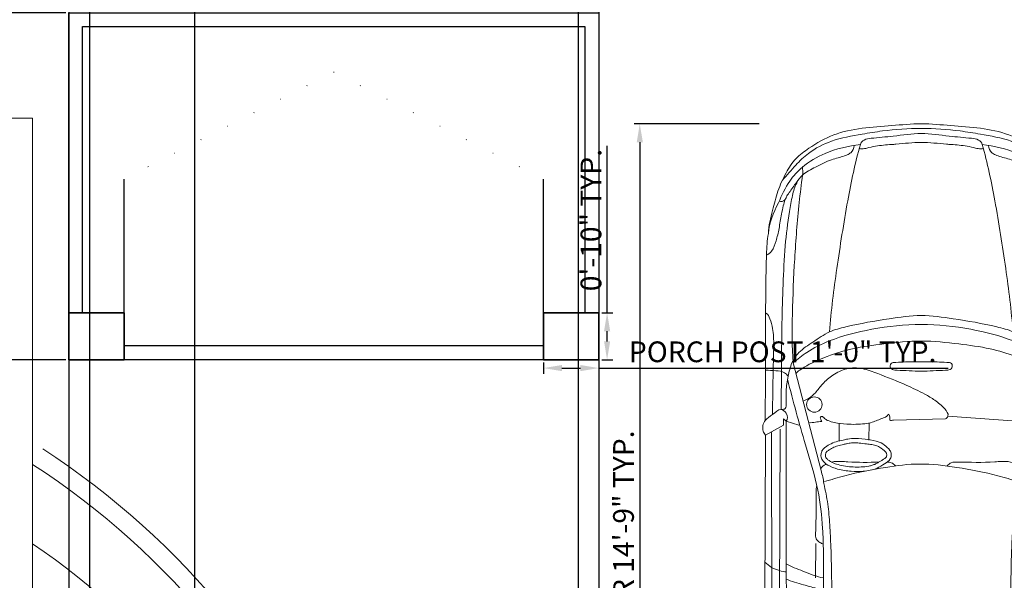
# Model space of a CAD drawing. Units: inches. Extents: x 1239 to 2276906, y 2273 to 321338.
# Tile 9 of 23: x 1541 to 1754, y 2507 to 2629. Entities that reach past the tile are written whole.
import ezdxf

# ---------------------------------------------------------------- set-up
doc = ezdxf.new("R2010")
doc.units = ezdxf.units.IN
doc.linetypes.add('DOT', pattern=[6.35, 0, -6.35])
for name, color, linetype, lineweight in [('A-ANNO-DIMS', 2, 'Continuous', 18), ('A-COLS', 7, 'Continuous', 35), ('A-FLOR-PORCH', 7, 'Continuous', 25), ('A-FLOR-PORCH-OVHD', 8, 'DOT', 18), ('C-PRKG', 8, 'Continuous', 13), ('L-PLNT', 94, 'Continuous', 13)]:
    doc.layers.add(name, color=color, linetype=linetype, lineweight=lineweight)
doc.styles.get("Standard").update_dxf_attribs({"font": 'arial.ttf'})
doc.dimstyles.new('ISO-25', dxfattribs={"dimtxt": 4.5, "dimasz": 4, "dimexe": 1.25, "dimexo": 0.625, "dimtad": 1, "dimdec": 1, "dimlunit": 3, "dimtxsty": 'Standard', "dimcen": 2.5, "dimadec": 0, "dimazin": 0, "dimtfac": 1, "dimtdec": 1, "dimtmove": 0, "dimatfit": 3, "dimfxl": 1, "dimarcsym": 0})

# ---------------------------------------------------------------- blocks, each defined once
blk = doc.blocks.new('A$C242571DA')
for p, q in [((1714.3, 1732.5), (3817.1, 1739.9)), ((1659.9, 1632), (1714.3, 1732.5)), ((1699.9, 1699.4), (2984.7, 1695.8)), ((1638.3, 1618.5), (1625.1, 1632)), ((1625.1, 1632), (1659.9, 1632)), ((1681.8, 1651.6), (2695.2, 1655.3)), ((1317.4, 1579.7), (1909.8, 1424.9)), ((1638.3, 1618.5), (2503.3, 1618.5)), ((1659.9, 1548.1), (1638.3, 1618.5)), ((2503.3, 1618.5), (2861.6, 1607.5)), ((3007.2, 1526.5), (2808.1, 1525.2)), ((1644, 1489.1), (1610.4, 1020.2)), ((2311.9, 1454.3), (2500.6, 1456.9)), ((3474.6, 1401.1), (3474.6, 843)), ((4315.2, 1398), (4377.3, 1370.5)), ((1626.1, 1006.5), (1632.8, 719.7)), ((3474.6, 345.6), (3474.6, 903.8)), ((1740.2, 584.9), (1649.3, 586.9)), ((1746.1, 420.6), (1649.3, 420.6)), ((4315.2, 348.7), (4377.3, 376.3)), ((1317.4, 167), (1909.8, 321.9)), ((2311.9, 292.5), (2500.6, 289.8)), ((3007.2, 220.3), (2808.1, 221.6)), ((1659.9, 198.7), (1638.3, 128.2)), ((1638.3, 128.2), (1625.1, 114.7)), ((1625.1, 114.7), (1659.9, 114.7)), ((1638.3, 128.2), (2503.3, 128.2)), ((1659.9, 114.7), (1714.3, 14.2)), ((2503.3, 128.2), (2861.6, 139.2)), ((1681.8, 95.1), (2695.2, 91.4)), ((1699.9, 47.3), (2984.7, 51)), ((1714.3, 14.2), (3817.1, 6.9))]:
    blk.add_line(p, q)
for centre in [(1546.4, 1462.5), (1546.4, 284.2)]:
    blk.add_ellipse(centre, major_axis=(0, 42.9), ratio=0.983266, start_param=4.712389, end_param=10.995574)
for points, knots in [([(1714.3, 1732.5), (1707.7, 1737.6), (1683.3, 1753), (1628.7, 1741.2), (1605.6, 1691.5), (1561.7, 1652.4), (1594.1, 1610.3), (1627.9, 1608.3), (1638.3, 1618.5)], [0, 0, 0, 0, 0.024864, 0.0846267, 0.1362471, 0.1900683, 0.2245199, 0.2681841, 0.2681841, 0.2681841, 0.2681841]), ([(3356.5, 1739.4), (3354.9, 1719.2), (3360.8, 1678.2), (3324, 1631.5), (3255.4, 1544.3), (3187.1, 1476.2), (3125.2, 1432.2)], [0, 0, 0, 0, 0.0597371, 0.1139981, 0.1672498, 0.3938869, 0.3938869, 0.3938869, 0.3938869]), ([(3745.3, 1736.8), (3748.5, 1730.1), (3764.2, 1717.1), (3811.5, 1698.6), (3894.7, 1686.7), (4002.9, 1663.2), (4107.9, 1648.7), (4195.8, 1638.3), (4258.6, 1603.2), (4302.1, 1549.7), (4339.9, 1483.8), (4365.2, 1407.6), (4389.6, 1324.4), (4397.9, 1266.9), (4401.8, 1235.2)], [0, 0, 0, 0, 0.0219205, 0.0572122, 0.1522539, 0.2718866, 0.3894011, 0.4710097, 0.5346344, 0.5986698, 0.6733118, 0.758696, 0.8351341, 0.9293726, 0.9293726, 0.9293726, 0.9293726]), ([(3817.1, 1739.9), (3833.2, 1729.7), (3882.9, 1718.2), (3973.3, 1695.2), (4085.1, 1680.5), (4193.8, 1662.8), (4280.6, 1644.3), (4343.9, 1598.1), (4390, 1540.3), (4427.4, 1448.7), (4457.8, 1336.6), (4475.7, 1233.4), (4478.4, 1175.1), (4479.3, 1161.6)], [0, 0, 0, 0, 0.056668, 0.14946, 0.28161, 0.392935, 0.481686, 0.542967, 0.622845, 0.69797, 0.833643, 0.965665, 1.00577, 1.00577, 1.00577, 1.00577]), ([(0, 873.4), (0, 927.8), (15.6, 1088.6), (25.5, 1309.8), (120.7, 1476.4), (189.2, 1569), (273.5, 1623.1), (369.9, 1666.3), (483, 1694.7), (561.3, 1714.9), (604.6, 1715.7)], [0, 0, 0, 0, 0.16039, 0.479033, 0.632967, 0.722015, 0.817474, 0.927562, 1.03733, 1.167094, 1.167094, 1.167094, 1.167094]), ([(604.6, 1715.7), (545.5, 1714.5), (448.5, 1664.6), (320.8, 1610.6), (225.4, 1521.2), (147.3, 1390.5), (121.7, 1275.2), (113.6, 1208.7)], [0, 0, 0, 0, 0.1772572, 0.3124951, 0.4151678, 0.5597243, 0.7575412, 0.7575412, 0.7575412, 0.7575412]), ([(722.7, 1726.6), (720.8, 1714.9), (694.5, 1689.9), (643, 1671.8), (573.6, 1655.4), (508.5, 1647), (455.2, 1634.7), (428.7, 1627.3), (416.9, 1624.1)], [0, 0, 0, 0, 0.034703, 0.0959761, 0.1659336, 0.2471559, 0.2929944, 0.3295918, 0.3295918, 0.3295918, 0.3295918]), ([(604.6, 1715.7), (642.1, 1723.4), (788.5, 1729.2), (1039.3, 1732.2), (1344.5, 1729.9), (1542, 1733.1), (1633.8, 1733.7)], [0, 0, 0, 0, 0.114897, 0.437061, 0.754269, 1.029686, 1.029686, 1.029686, 1.029686]), ([(1043.6, 1729.2), (1048.6, 1717.9), (1080.9, 1704.2), (1138.6, 1687.6), (1237.7, 1685.6), (1394.7, 1691.3), (1521.7, 1692.4), (1601.5, 1692.7)], [0, 0, 0, 0, 0.0364992, 0.0923739, 0.1867837, 0.3273982, 0.5667068, 0.5667068, 0.5667068, 0.5667068]), ([(1356.8, 1732.2), (1357.1, 1712.8), (1360, 1678.8), (1363.9, 1630.5), (1383.3, 1613.5), (1391, 1607.2)], [0, 0, 0, 0, 1.462159, 2.651105, 3.386321, 3.386321, 3.386321, 3.386321]), ([(2414.7, 1735), (2424.9, 1723.3), (2447.2, 1698.8), (2461.2, 1657.6), (2468.1, 1629), (2468, 1616.1)], [1.808086, 1.808086, 1.808086, 1.808086, 2.918874, 4.131288, 5.10151, 5.10151, 5.10151, 5.10151]), ([(2984.7, 1695.8), (3051, 1695.6), (3172.1, 1691.3), (3367.4, 1677.6), (3575.2, 1664.3), (3788.2, 1643.6), (3968, 1628.1), (4103.8, 1616.8), (4203.6, 1578.1), (4271.8, 1519.5), (4300.6, 1452.1), (4341.7, 1305.3), (4361.8, 1111.2), (4367.5, 936.8), (4367.5, 873.4)], [0, 0, 0, 0, 0.198873, 0.363323, 0.587433, 0.823543, 1.004622, 1.129816, 1.230113, 1.320655, 1.388577, 1.443334, 1.771447, 1.958652, 1.958652, 1.958652, 1.958652]), ([(310.7, 1637.3), (282.5, 1613.7), (230.1, 1569.9), (148.7, 1486.2), (84.8, 1361.3), (60, 1219), (32.6, 1054.3), (25.1, 944.9), (25.1, 873.4)], [0, 0, 0, 0, 0.1095129, 0.2035347, 0.3452507, 0.5161382, 0.6275464, 0.8383798, 0.8383798, 0.8383798, 0.8383798]), ([(426.8, 1656.7), (428.5, 1646.6), (426.9, 1625), (399.8, 1616.6), (368.1, 1593.9), (328, 1564.6), (271.6, 1523.9), (237, 1451.9), (196.2, 1376.7), (183.8, 1314.9), (170, 1279.6), (157.2, 1254.2), (133.3, 1244.4), (118.6, 1242.9)], [0, 0, 0, 0, 0.0304541, 0.0502818, 0.0786089, 0.1479133, 0.1986294, 0.2831705, 0.3780326, 0.4523267, 0.4667809, 0.4902599, 0.5347198, 0.5347198, 0.5347198, 0.5347198]), ([(323.7, 1557.5), (344.8, 1571.9), (400.4, 1585.1), (516, 1606.8), (680.3, 1625.8), (885.4, 1635.7), (1116.8, 1642.2), (1346.1, 1644.2), (1504.7, 1644.7), (1574, 1645.7)], [0, 0, 0, 0, 0.076148, 0.165903, 0.355672, 0.569871, 0.782325, 1.050047, 1.257936, 1.257936, 1.257936, 1.257936]), ([(1574, 1645.7), (1572.9, 1638), (1574.1, 1622), (1559.9, 1618.7), (1555.2, 1617.8)], [0, 0, 0, 0, 0.02274132, 0.03717479, 0.03717479, 0.03717479, 0.03717479]), ([(2695.2, 1655.3), (2829.9, 1655.3), (3041.2, 1651.4), (3351.3, 1630.7), (3527.5, 1623.2), (3626.6, 1612)], [0, 0, 0, 0, 0.4042759, 0.6333827, 0.9326252, 0.9326252, 0.9326252, 0.9326252]), ([(1317.4, 1579.7), (1227.8, 1586.1), (1036, 1584.8), (741.2, 1572.5), (486.1, 1553.3), (333.3, 1534.3), (283.3, 1528.5)], [0, 0, 0, 0, 0.269375, 0.574535, 0.885339, 1.036319, 1.036319, 1.036319, 1.036319]), ([(1555.2, 1617.8), (1527.7, 1617.8), (1472.5, 1620.4), (1392.7, 1608.8), (1318.5, 1591), (1249.4, 1545.5), (1201.4, 1466.7), (1142.8, 1385.7), (1104.8, 1240.4), (1076, 1072.3), (1056.4, 932.4), (1056.4, 873.4)], [0, 0, 0, 0, 0.082256, 0.165174, 0.241383, 0.30939, 0.405348, 0.511507, 0.603349, 0.843635, 1.017671, 1.017671, 1.017671, 1.017671]), ([(1317.4, 1579.7), (1296.6, 1555.5), (1247.9, 1494.4), (1177.6, 1350.5), (1124.2, 1137.4), (1105.5, 964.9), (1105.5, 873.4)], [0, 0, 0, 0, 0.0947759, 0.2311242, 0.4700259, 0.7400315, 0.7400315, 0.7400315, 0.7400315]), ([(3535.9, 1563.1), (3520.1, 1550.9), (3484.4, 1526.1), (3408.2, 1510.9), (3323.4, 1473.1), (3207.9, 1445), (3072.6, 1422.2), (2866.9, 1404.6), (2626.4, 1412.9), (2396.7, 1410.8), (2200.9, 1416.9), (2001.3, 1438.2), (1732.1, 1525.9), (1527.9, 1578.9), (1407.5, 1610.7)], [0, 0, 0, 0, 0.05975, 0.126928, 0.230034, 0.336675, 0.482225, 0.641324, 0.954906, 1.203173, 1.330375, 1.542773, 1.802261, 2.175545, 2.175545, 2.175545, 2.175545]), ([(2424, 1618.7), (2441.5, 1589.9), (2464.2, 1518.9), (2495.4, 1450.9), (2501.6, 1411.3)], [0, 0, 0, 0, 0.1000351, 0.2184418, 0.2184418, 0.2184418, 0.2184418]), ([(2507.7, 1618.4), (2521, 1587.7), (2536.6, 1527.1), (2559.6, 1458.5), (2563.3, 1420.6), (2563.8, 1411.4)], [0, 0, 0, 0, 2.528586, 4.711885, 5.408215, 5.408215, 5.408215, 5.408215]), ([(2861.6, 1607.5), (2921.1, 1607.3), (3047.2, 1600.8), (3191.4, 1602), (3356.6, 1584.1), (3498.3, 1570.6), (3623.2, 1549.4), (3664.1, 1533.3)], [0, 0, 0, 0, 0.1783018, 0.3787173, 0.431954, 0.6762374, 0.8077184, 0.8077184, 0.8077184, 0.8077184]), ([(3248.1, 1545.2), (3226.9, 1550.4), (3176.1, 1562.1), (3113.7, 1592.9), (3052.6, 1605.3), (3010.4, 1578.8), (3010.3, 1545.3), (3010.3, 1515.9), (3033.7, 1500.1), (3052.6, 1465.2), (3078.9, 1443.5), (3084, 1424.4)], [0, 0, 0, 0, 0.0655106, 0.1550445, 0.2094604, 0.2438604, 0.287164, 0.3001388, 0.3275984, 0.3616951, 0.4200969, 0.4200969, 0.4200969, 0.4200969]), ([(3319, 1587.1), (3303.3, 1568.1), (3256.9, 1516.7), (3206.7, 1467.3), (3171.4, 1439.5)], [0, 0, 0, 0, 1.868162, 5.271297, 5.271297, 5.271297, 5.271297]), ([(3626.6, 1612), (3702.5, 1609.1), (3826.2, 1596.8), (3991.4, 1583.2), (4111.7, 1562.4), (4212.2, 1522.7), (4290.4, 1488), (4300.7, 1447.5)], [0, 0, 0, 0, 0.2277977, 0.3719478, 0.4996814, 0.5863441, 0.709615, 0.709615, 0.709615, 0.709615]), ([(1372.8, 1563.1), (1357.2, 1545), (1321.6, 1490.1), (1277, 1385.7), (1232.8, 1244.2), (1211.1, 1069.4), (1196.8, 942.4), (1196.8, 873.4)], [0, 0, 0, 0, 0.0708922, 0.1925846, 0.3348457, 0.5072814, 0.7109928, 0.7109928, 0.7109928, 0.7109928]), ([(2808.1, 1525.2), (2791.9, 1525.1), (2751.9, 1519.7), (2710.6, 1472.6), (2690, 1431.1), (2690.5, 1409.6)], [0, 0, 0, 0, 0.0486628, 0.1144515, 0.1777721, 0.1777721, 0.1777721, 0.1777721]), ([(3275.5, 1532.8), (3287.5, 1528.3), (3299.8, 1504.9), (3308.4, 1482.5), (3311.7, 1472.6)], [0, 0, 0, 0, 0.983949, 1.771691, 1.771691, 1.771691, 1.771691]), ([(3372.2, 1495.3), (3354.4, 1496.8), (3316, 1494.7), (3291.6, 1525.8), (3275.5, 1532.8)], [0, 0, 0, 0, 0.0535488, 0.1060573, 0.1060573, 0.1060573, 0.1060573]), ([(3664.1, 1533.3), (3687, 1526), (3734.8, 1502.3), (3816.7, 1444.8), (3884.1, 1342.9), (3925.1, 1239.9), (3937.3, 1177), (3940.4, 1157.6)], [0, 0, 0, 0, 0.0720749, 0.1581284, 0.2958089, 0.4262456, 0.4842292, 0.4842292, 0.4842292, 0.4842292]), ([(1898.5, 1426.2), (1889, 1420.6), (1871, 1397.2), (1856.4, 1345.2), (1867.7, 1233.5), (1864.3, 1132.3), (1863, 1038.5), (1876.9, 1022.3), (1884.5, 1015.7)], [0, 0, 0, 0, 0.842998, 2.122875, 3.997599, 9.174838, 10.012722, 10.751336, 10.751336, 10.751336, 10.751336]), ([(1909.8, 1424.9), (1933.5, 1418.7), (1995.6, 1407.6), (2094.4, 1385.8), (2211.8, 1377.1), (2419, 1366.9), (2704.7, 1366.5), (3032.7, 1354.2), (3316.2, 1371), (3558.7, 1415.9), (3789.1, 1461.7), (4028.9, 1452.9), (4196.2, 1455.2), (4292.7, 1447.9), (4300.7, 1447.5)], [0, 0, 0, 0, 0.073325, 0.188896, 0.303039, 0.425821, 0.811242, 1.159737, 1.41058, 1.660623, 1.899627, 2.11145, 2.377727, 2.401703, 2.401703, 2.401703, 2.401703]), ([(1997.2, 1450.5), (2039.7, 1454.5), (2126.7, 1451.9), (2219.8, 1454.5), (2287.1, 1456.9), (2305.7, 1434.4), (2313.2, 1419.9), (2315.8, 1413.5)], [0, 0, 0, 0, 3.267856, 6.568708, 7.399663, 8.099385, 8.621705, 8.621705, 8.621705, 8.621705]), ([(113.6, 1208.7), (215.2, 1238.6), (443.2, 1284.9), (788, 1338.7), (1029.5, 1370.7), (1146.4, 1378.6)], [0, 0, 0, 0, 0.317374, 0.69576, 1.04714, 1.04714, 1.04714, 1.04714]), ([(1969.6, 1407.3), (1960.5, 1369.8), (1927, 1259.1), (1890.9, 1078.4), (1874.3, 933), (1874.3, 864.4)], [0, 0, 0, 0, 0.1139079, 0.3411539, 0.543502, 0.543502, 0.543502, 0.543502]), ([(3231.5, 1368.3), (3240.8, 1356.2), (3253.1, 1315.7), (3271.9, 1240.7), (3297.9, 1127.9), (3310.5, 974.6), (3311.2, 858.3), (3311.6, 794.4)], [0, 0, 0, 0, 0.0451009, 0.1211996, 0.2308505, 0.385263, 0.5739042, 0.5739042, 0.5739042, 0.5739042]), ([(3294.8, 1174.5), (3294.8, 1207.4), (3299.6, 1249.5), (3298.3, 1303.9), (3326.3, 1329), (3363.9, 1320.7), (3399.3, 1329.3), (3422.1, 1315.7), (3430.7, 1297.9), (3438.7, 1234.2), (3439.6, 1174.4), (3434.7, 1112.2), (3418.9, 1102), (3395.9, 1098.6), (3362.6, 1100.9), (3331.1, 1096.6), (3298.8, 1107.6), (3297.3, 1140.3), (3294.8, 1160.9), (3294.8, 1174.5)], [0, 0, 0, 0, 0.0969044, 0.1295913, 0.1506192, 0.1985921, 0.2360698, 0.2557908, 0.2719711, 0.2929882, 0.44406, 0.4519132, 0.4720918, 0.4918599, 0.5228758, 0.5707096, 0.5892096, 0.6145759, 0.654681, 0.654681, 0.654681, 0.654681]), ([(113.6, 1208.7), (103.3, 1207), (83.6, 1187.6), (76.5, 1122.2), (68.2, 1017.3), (53.4, 925), (53.4, 873.4)], [0, 0, 0, 0, 0.0314754, 0.0702057, 0.1915753, 0.3439346, 0.3439346, 0.3439346, 0.3439346]), ([(135.5, 1213.1), (139.1, 1211.8), (138.4, 1193.3), (132.6, 1168.3), (118.8, 1111.9), (115.6, 1058.9), (109, 974.6), (102.4, 920.1), (102.4, 873.4)], [0, 0, 0, 0, 0.0114788, 0.0403472, 0.0875838, 0.1755608, 0.1991501, 0.3369659, 0.3369659, 0.3369659, 0.3369659]), ([(4401.8, 1235.2), (4411.9, 1185.3), (4421.6, 1065.8), (4424.1, 946.5), (4424.1, 878)], [0, 0, 0, 0, 0.1502861, 0.3522699, 0.3522699, 0.3522699, 0.3522699]), ([(3940.4, 1157.6), (3949.9, 1111), (3964.3, 1016.4), (3960.5, 921), (3959.8, 873.4)], [0, 0, 0, 0, 0.140379, 0.2808468, 0.2808468, 0.2808468, 0.2808468]), ([(3339.2, 1099), (3339.1, 1094.8), (3336.4, 1010.6), (3333.2, 926.3), (3330, 846.2)], [11.235438, 11.235438, 11.235438, 11.235438, 11.552536, 17.586883, 17.586883, 17.586883, 17.586883]), ([(1311.3, 873.4), (1311.2, 902.4), (1309.2, 950.9), (1315, 1002.2), (1314.2, 1039.4), (1332.1, 1044.9), (1345.7, 1044.2), (1356.8, 1028.5), (1359.2, 970.2), (1361.5, 917.6), (1362.9, 873.4)], [0, 0, 0, 0, 0.0857277, 0.1381048, 0.1641986, 0.1769751, 0.1890325, 0.2028129, 0.2286049, 0.3592554, 0.3592554, 0.3592554, 0.3592554]), ([(1626.1, 1006.5), (1623.5, 1013), (1603.1, 1029.4), (1559.1, 995), (1523, 951.9), (1480.3, 878.3), (1430.5, 774.3), (1385.5, 658.5), (1343.7, 551.3), (1343, 461.7), (1380.3, 386.9), (1428.2, 329.9), (1480.1, 294.6), (1509.8, 257.4), (1524.8, 232.6), (1528, 222.1)], [0, 0, 0, 0, 0.527288, 1.647451, 3.487558, 5.099073, 7.968657, 12.238313, 14.475187, 16.613757, 18.744202, 20.639343, 22.223389, 23.452731, 24.286529, 24.286529, 24.286529, 24.286529]), ([(3231.5, 378.5), (3240.8, 390.5), (3253.1, 431), (3271.9, 506.1), (3297.9, 618.9), (3310.5, 772.1), (3311.2, 888.4), (3311.6, 952.4)], [0, 0, 0, 0, 0.0451009, 0.1211996, 0.2308505, 0.385263, 0.5739042, 0.5739042, 0.5739042, 0.5739042]), ([(0, 873.4), (0, 819), (15.6, 658.1), (25.5, 437), (120.7, 270.3), (189.2, 177.8), (273.5, 123.7), (369.9, 80.4), (483, 52), (561.3, 31.9), (604.6, 31)], [0, 0, 0, 0, 0.16039, 0.479033, 0.632967, 0.722015, 0.817474, 0.927562, 1.03733, 1.167094, 1.167094, 1.167094, 1.167094]), ([(310.7, 109.5), (282.5, 133.1), (230.1, 176.9), (148.7, 260.5), (84.8, 385.5), (60, 527.8), (32.6, 692.4), (25.1, 801.9), (25.1, 873.4)], [0, 0, 0, 0, 0.1095129, 0.2035347, 0.3452507, 0.5161382, 0.6275464, 0.8383798, 0.8383798, 0.8383798, 0.8383798]), ([(113.6, 538.1), (103.3, 539.8), (83.6, 559.2), (76.5, 624.5), (68.2, 729.4), (53.4, 821.7), (53.4, 873.4)], [0, 0, 0, 0, 0.0314754, 0.0702057, 0.1915753, 0.3439346, 0.3439346, 0.3439346, 0.3439346]), ([(135.5, 533.6), (139.1, 534.9), (138.4, 553.4), (132.6, 578.4), (118.8, 634.9), (115.6, 687.8), (109, 772.2), (102.4, 826.7), (102.4, 873.4)], [0, 0, 0, 0, 0.0114788, 0.0403472, 0.0875838, 0.1755608, 0.1991501, 0.3369659, 0.3369659, 0.3369659, 0.3369659]), ([(1555.2, 129), (1527.7, 129), (1472.5, 126.3), (1392.7, 138), (1318.5, 155.7), (1249.4, 201.3), (1201.4, 280.1), (1142.8, 361.1), (1104.8, 506.4), (1076, 674.5), (1056.4, 814.4), (1056.4, 873.4)], [0, 0, 0, 0, 0.082256, 0.165174, 0.241383, 0.30939, 0.405348, 0.511507, 0.603349, 0.843635, 1.017671, 1.017671, 1.017671, 1.017671]), ([(1317.4, 167), (1296.6, 191.2), (1247.9, 252.4), (1177.6, 396.3), (1124.2, 609.4), (1105.5, 781.8), (1105.5, 873.4)], [0, 0, 0, 0, 0.0947759, 0.2311242, 0.4700259, 0.7400315, 0.7400315, 0.7400315, 0.7400315]), ([(1372.8, 183.6), (1357.2, 201.8), (1321.6, 256.7), (1277, 361), (1232.8, 502.6), (1211.1, 677.3), (1196.8, 804.3), (1196.8, 873.4)], [0, 0, 0, 0, 0.0708922, 0.1925846, 0.3348457, 0.5072814, 0.7109928, 0.7109928, 0.7109928, 0.7109928]), ([(1311.3, 873.4), (1311.2, 844.3), (1309.2, 795.8), (1315, 744.6), (1314.2, 707.4), (1332.1, 701.9), (1345.7, 702.6), (1356.8, 718.2), (1359.2, 776.6), (1361.5, 829.1), (1362.9, 873.4)], [0, 0, 0, 0, 0.0857277, 0.1381048, 0.1641986, 0.1769751, 0.1890325, 0.2028129, 0.2286049, 0.3592554, 0.3592554, 0.3592554, 0.3592554]), ([(2984.7, 51), (3051, 51.1), (3172.1, 55.5), (3367.4, 69.2), (3575.2, 82.5), (3788.2, 103.1), (3968, 118.7), (4103.8, 130), (4203.6, 168.6), (4271.8, 227.3), (4300.6, 294.7), (4341.7, 441.5), (4361.8, 635.5), (4367.5, 809.9), (4367.5, 873.4)], [0, 0, 0, 0, 0.198873, 0.363323, 0.587433, 0.823543, 1.004622, 1.129816, 1.230113, 1.320655, 1.388577, 1.443334, 1.771447, 1.958652, 1.958652, 1.958652, 1.958652]), ([(3339.2, 647.8), (3339.1, 652), (3336.4, 736.2), (3333.2, 820.5), (3330, 900.6)], [11.235438, 11.235438, 11.235438, 11.235438, 11.552536, 17.586883, 17.586883, 17.586883, 17.586883]), ([(3940.4, 589.1), (3949.9, 635.7), (3964.3, 730.4), (3960.5, 825.8), (3959.8, 873.4)], [0, 0, 0, 0, 0.140379, 0.2808468, 0.2808468, 0.2808468, 0.2808468]), ([(4401.8, 511.5), (4411.9, 561.5), (4421.6, 681), (4424.1, 800.3), (4424.1, 868.8)], [0, 0, 0, 0, 0.1502861, 0.3522699, 0.3522699, 0.3522699, 0.3522699]), ([(1969.6, 339.5), (1960.5, 377), (1926.9, 487.6), (1892.9, 662.7), (1874.3, 801.8), (1874.3, 864.4)], [0, 0, 0, 0, 0.1139079, 0.3411539, 0.5260188, 0.5260188, 0.5260188, 0.5260188]), ([(1639.2, 326.1), (1635.3, 323.6), (1629, 318.4), (1613.1, 314.9), (1612, 324.2), (1613.2, 330.4), (1619, 337.5), (1629, 345.7), (1637.9, 366.1), (1649, 404.8), (1656.3, 472.9), (1656.2, 543.1), (1644.6, 610.9), (1623, 651.2), (1615, 684.3), (1598.5, 691.2), (1604, 696.6), (1610.3, 699.7), (1618.8, 698.9), (1625.9, 701.3), (1638.1, 698.6), (1633, 713.4), (1632.8, 719.7)], [0, 0, 0, 0, 0.0138597, 0.0278304, 0.0329137, 0.0379971, 0.0465756, 0.0592704, 0.0762214, 0.1105991, 0.1789801, 0.2766959, 0.3173629, 0.3800771, 0.4110544, 0.4160421, 0.4210284, 0.4277212, 0.4387433, 0.4448131, 0.4508005, 0.4694463, 0.4694463, 0.4694463, 0.4694463]), ([(1740.2, 584.9), (1737.8, 571.7), (1749.5, 644.3), (1766.4, 664.5), (1792.2, 700.2), (1821.5, 709.7), (1853.1, 703.9), (1874, 668.4), (1904.5, 622.6), (1915.6, 557.2), (1915.1, 484.2), (1905.7, 417.6), (1884.9, 362.8), (1859.3, 329.1), (1831.3, 318.1), (1810.8, 322.7), (1792.2, 329.3), (1777.9, 350.3), (1753, 385.9), (1737.9, 465.8), (1728.8, 497.3), (1742.4, 597.6), (1740.2, 584.9)], [0, 0, 0, 0, 0.03969, 0.089634, 0.13125, 0.1542862, 0.1797268, 0.2207266, 0.2680991, 0.3447665, 0.4095645, 0.4843001, 0.541515, 0.5817687, 0.6060665, 0.6262474, 0.6436722, 0.6634686, 0.6988791, 0.7758465, 0.8696394, 0.907731, 0.907731, 0.907731, 0.907731]), ([(1863.4, 685.6), (1863.6, 693.5), (1865.3, 711), (1876.9, 724.5), (1884.5, 731)], [9.436432, 9.436432, 9.436432, 9.436432, 10.012722, 10.751336, 10.751336, 10.751336, 10.751336]), ([(1764.9, 587), (1765.6, 590.8), (1766.4, 595.5), (1768.5, 605.7), (1769.7, 611.3), (1773.4, 626.6), (1775.6, 633), (1779.7, 642.1), (1781.6, 644.9), (1785.7, 650.6), (1787.1, 652.5), (1793, 660.3), (1797.4, 666.2), (1804.2, 673.7), (1806.8, 676.1), (1811.1, 679.4), (1812.9, 680.5), (1816.8, 682.1), (1818.8, 682.7), (1824.4, 683.5), (1828.3, 683.2), (1832.5, 682), (1833.6, 681.5), (1836, 680.2), (1837.9, 678.7), (1842.4, 673.7), (1844.9, 670.1), (1850.3, 661.7), (1853.4, 656.6), (1859.3, 647.3), (1862.1, 642.8), (1868.3, 632.6), (1871.4, 626.9), (1876.7, 615.7), (1878.9, 609.8), (1882.8, 597.4), (1884.4, 590.8), (1888.3, 570.5), (1889.7, 556.1), (1891.2, 527.4), (1891.1, 513.1), (1888.9, 470), (1885.1, 441.2), (1874.3, 404), (1870.6, 393.8), (1863.5, 378.7), (1860.6, 373.4), (1854.4, 363.6), (1851.2, 359.2), (1845, 352.6), (1842, 350.2), (1835.8, 346.4), (1832.6, 345.3), (1828.8, 344.6), (1827.9, 344.6), (1824.6, 344.9), (1822.6, 345.2), (1817.8, 346.4), (1814.9, 347.3), (1810.9, 348.7), (1809.4, 349.4), (1808.3, 350.1), (1808.1, 350.2), (1807.3, 351), (1806.7, 351.6), (1804.7, 354), (1803.1, 356.2), (1799.6, 361.3), (1798, 363.7), (1794.9, 368.2), (1793.4, 370.4), (1789.2, 376.9), (1786.7, 381), (1782.4, 389.3), (1780.5, 393.6), (1776.9, 403), (1775.2, 408), (1770.7, 423.5), (1768.3, 434.2), (1764.9, 450.5), (1763.6, 456.4), (1761.4, 466.8), (1760.4, 471.4), (1758.1, 484.4), (1757.3, 492.6), (1757.5, 510.7), (1757.8, 516.5), (1758.6, 528.4), (1759.1, 534.3), (1761.1, 553.9), (1763.1, 570.6), (1764.4, 581.5), (1764.6, 583), (1764.7, 585), (1764.8, 585.5), (1764.8, 586.5), (1764.8, 586.7), (1764.9, 587)], [0.497033, 0.497033, 0.497033, 0.497033, 0.723444, 0.723444, 0.974636, 0.974636, 1.50964, 1.50964, 2.044645, 2.044645, 2.271061, 2.271061, 2.862376, 2.862376, 3.217654, 3.217654, 3.537253, 3.537253, 3.856852, 3.856852, 4.368613, 4.368613, 4.584627, 4.584627, 4.99269, 4.99269, 5.400753, 5.400753, 5.808816, 5.808816, 6.216879, 6.216879, 6.778716, 6.778716, 7.350371, 7.350371, 7.922025, 7.922025, 9.065335, 9.065335, 10.208644, 10.208644, 12.495263, 12.495263, 13.409896, 13.409896, 13.929088, 13.929088, 14.44828, 14.44828, 14.909885, 14.909885, 15.371489, 15.371489, 15.62524, 15.62524, 15.87899, 15.87899, 16.120875, 16.120875, 16.36276, 16.36276, 16.51635, 16.51635, 16.669941, 16.669941, 16.921521, 16.921521, 17.136676, 17.136676, 17.351831, 17.351831, 17.782142, 17.782142, 18.204974, 18.204974, 18.627807, 18.627807, 19.473473, 19.473473, 19.978923, 19.978923, 20.484372, 20.484372, 21.475119, 21.475119, 21.859144, 21.859144, 22.162884, 22.162884, 22.770362, 22.770362, 22.900493, 22.900493, 22.951221, 22.951221, 22.964298, 22.964298, 22.964298, 22.964298]), ([(1863.7, 379.4), (1862.6, 384.2), (1857.6, 413.7), (1866.5, 501.6), (1865.2, 581.4), (1864.1, 639.5)], [1.749253, 1.749253, 1.749253, 1.749253, 2.122875, 3.997599, 8.307432, 8.307432, 8.307432, 8.307432]), ([(3294.8, 572.3), (3294.8, 539.4), (3299.6, 497.2), (3298.3, 442.9), (3326.3, 417.8), (3363.9, 426), (3399.3, 417.5), (3422.1, 431), (3430.7, 448.9), (3438.7, 512.5), (3439.6, 572.4), (3434.7, 634.6), (3418.9, 644.7), (3395.9, 648.2), (3362.6, 645.9), (3331.1, 650.1), (3298.8, 639.2), (3297.3, 606.5), (3294.8, 585.9), (3294.8, 572.3)], [0, 0, 0, 0, 0.0969044, 0.1295913, 0.1506192, 0.1985921, 0.2360698, 0.2557908, 0.2719711, 0.2929882, 0.44406, 0.4519132, 0.4720918, 0.4918599, 0.5228758, 0.5707096, 0.5892096, 0.6145759, 0.654681, 0.654681, 0.654681, 0.654681]), ([(3664.1, 213.5), (3687, 220.8), (3734.8, 244.4), (3816.7, 302), (3884.1, 403.8), (3925.1, 506.9), (3937.3, 569.7), (3940.4, 589.1)], [0, 0, 0, 0, 0.0720749, 0.1581284, 0.2958089, 0.4262456, 0.4842292, 0.4842292, 0.4842292, 0.4842292]), ([(3817.1, 6.9), (3833.2, 17), (3882.9, 28.6), (3973.3, 51.5), (4085.1, 66.3), (4193.8, 84), (4280.6, 102.4), (4343.9, 148.6), (4390, 206.4), (4427.4, 298), (4457.8, 410.1), (4475.7, 513.3), (4478.4, 571.6), (4479.3, 585.2)], [0, 0, 0, 0, 0.056668, 0.14946, 0.28161, 0.392935, 0.481686, 0.542967, 0.622845, 0.69797, 0.833643, 0.965665, 1.00577, 1.00577, 1.00577, 1.00577]), ([(604.6, 31), (545.5, 32.3), (448.5, 82.2), (320.8, 136.1), (225.4, 225.5), (147.3, 356.2), (121.7, 471.5), (113.6, 538.1)], [0, 0, 0, 0, 0.1772572, 0.3124951, 0.4151678, 0.5597243, 0.7575412, 0.7575412, 0.7575412, 0.7575412]), ([(113.6, 538.1), (215.2, 508.2), (443.2, 461.9), (788, 408.1), (1029.5, 376), (1146.4, 368.2)], [0, 0, 0, 0, 0.317374, 0.69576, 1.04714, 1.04714, 1.04714, 1.04714]), ([(426.8, 90), (428.5, 100.2), (426.9, 121.8), (399.8, 130.1), (368.1, 152.8), (328, 182.2), (271.6, 222.8), (237, 294.9), (196.2, 370.1), (183.8, 431.9), (170, 467.2), (157.2, 492.6), (133.3, 502.4), (118.6, 503.9)], [0, 0, 0, 0, 0.0304541, 0.0502818, 0.0786089, 0.1479133, 0.1986294, 0.2831705, 0.3780326, 0.4523267, 0.4667809, 0.4902599, 0.5347198, 0.5347198, 0.5347198, 0.5347198]), ([(3745.3, 10), (3748.5, 16.7), (3764.2, 29.7), (3811.5, 48.1), (3894.7, 60.1), (4002.9, 83.6), (4107.9, 98), (4195.8, 108.4), (4258.6, 143.5), (4302.1, 197), (4339.9, 262.9), (4365.2, 339.2), (4389.6, 422.4), (4397.9, 479.8), (4401.8, 511.5)], [0, 0, 0, 0, 0.0219205, 0.0572122, 0.1522539, 0.2718866, 0.3894011, 0.4710097, 0.5346344, 0.5986698, 0.6733118, 0.758696, 0.8351341, 0.9293726, 0.9293726, 0.9293726, 0.9293726]), ([(1909.8, 321.9), (1933.5, 328.1), (1995.6, 339.2), (2094.4, 361), (2211.8, 369.6), (2419, 379.8), (2704.7, 380.3), (3032.7, 392.6), (3316.2, 375.8), (3558.7, 330.9), (3789.1, 285.1), (4028.9, 293.9), (4196.2, 291.5), (4292.7, 298.8), (4300.7, 299.2)], [0, 0, 0, 0, 0.073325, 0.188896, 0.303039, 0.425821, 0.811242, 1.159737, 1.41058, 1.660623, 1.899627, 2.11145, 2.377727, 2.401703, 2.401703, 2.401703, 2.401703]), ([(3535.9, 183.7), (3520.1, 195.9), (3484.4, 220.6), (3408.2, 235.8), (3323.4, 273.7), (3207.9, 301.8), (3072.6, 324.6), (2866.9, 342.1), (2626.4, 333.8), (2396.7, 335.9), (2200.9, 329.9), (2001.3, 308.6), (1732.1, 220.8), (1527.9, 167.8), (1407.5, 136)], [0, 0, 0, 0, 0.05975, 0.126928, 0.230034, 0.336675, 0.482225, 0.641324, 0.954906, 1.203173, 1.330375, 1.542773, 1.802261, 2.175545, 2.175545, 2.175545, 2.175545]), ([(1898.5, 320.6), (1889, 326.2), (1880.8, 336.8), (1874.8, 348.3), (1874, 349.7)], [0, 0, 0, 0, 0.8429982, 0.9626806, 0.9626806, 0.9626806, 0.9626806]), ([(1997.2, 296.3), (2039.7, 292.2), (2126.7, 294.9), (2219.8, 292.3), (2287.1, 289.9), (2305.7, 312.3), (2313.2, 326.9), (2315.8, 333.2)], [0, 0, 0, 0, 3.267856, 6.568708, 7.399663, 8.099385, 8.621705, 8.621705, 8.621705, 8.621705]), ([(2424, 128), (2441.5, 156.9), (2464.2, 227.8), (2495.4, 295.8), (2501.6, 335.5)], [0, 0, 0, 0, 0.1000351, 0.2184418, 0.2184418, 0.2184418, 0.2184418]), ([(2507.7, 128.3), (2521, 159.1), (2536.6, 219.7), (2559.6, 288.3), (2563.3, 326.1), (2563.8, 335.3)], [0, 0, 0, 0, 2.528586, 4.711885, 5.408215, 5.408215, 5.408215, 5.408215]), ([(2808.1, 221.6), (2791.9, 221.6), (2751.9, 227.1), (2710.6, 274.2), (2690, 315.7), (2690.5, 337.1)], [0, 0, 0, 0, 0.0486628, 0.1144515, 0.1777721, 0.1777721, 0.1777721, 0.1777721]), ([(3248.1, 201.6), (3226.9, 196.3), (3176.1, 184.7), (3113.7, 153.8), (3052.6, 141.4), (3010.4, 168), (3010.3, 201.5), (3010.3, 230.9), (3033.7, 246.6), (3052.6, 281.6), (3078.9, 303.2), (3084, 322.4)], [0, 0, 0, 0, 0.0655106, 0.1550445, 0.2094604, 0.2438604, 0.287164, 0.3001388, 0.3275984, 0.3616951, 0.4200969, 0.4200969, 0.4200969, 0.4200969]), ([(3356.5, 7.4), (3354.9, 27.5), (3360.8, 68.5), (3324, 115.2), (3255.4, 202.5), (3187.1, 270.5), (3125.2, 314.6)], [0, 0, 0, 0, 0.0597371, 0.1139981, 0.1672498, 0.3938869, 0.3938869, 0.3938869, 0.3938869]), ([(3319, 159.7), (3303.3, 178.6), (3256.9, 230), (3206.7, 279.5), (3171.4, 307.2)], [0, 0, 0, 0, 1.868162, 5.271297, 5.271297, 5.271297, 5.271297]), ([(3275.5, 214), (3287.5, 218.5), (3299.8, 241.9), (3308.4, 264.3), (3311.7, 274.2)], [0, 0, 0, 0, 0.983949, 1.771691, 1.771691, 1.771691, 1.771691]), ([(3626.6, 134.7), (3702.5, 137.7), (3826.2, 149.9), (3991.4, 163.5), (4111.7, 184.4), (4212.2, 224.1), (4290.4, 258.8), (4300.7, 299.2)], [0, 0, 0, 0, 0.2277977, 0.3719478, 0.4996814, 0.5863441, 0.709615, 0.709615, 0.709615, 0.709615]), ([(1317.4, 167), (1227.8, 160.7), (1036, 161.9), (741.2, 174.2), (486.1, 193.4), (333.3, 212.5), (283.3, 218.3)], [0, 0, 0, 0, 0.269375, 0.574535, 0.885339, 1.036319, 1.036319, 1.036319, 1.036319]), ([(3372.2, 251.5), (3354.4, 249.9), (3316, 252), (3291.6, 220.9), (3275.5, 214)], [0, 0, 0, 0, 0.0535488, 0.1060573, 0.1060573, 0.1060573, 0.1060573]), ([(323.7, 189.2), (344.8, 174.9), (400.4, 161.7), (516, 139.9), (680.3, 121), (885.4, 111), (1116.8, 104.5), (1346.1, 102.5), (1504.7, 102), (1574, 101.1)], [0, 0, 0, 0, 0.076148, 0.165903, 0.355672, 0.569871, 0.782325, 1.050047, 1.257936, 1.257936, 1.257936, 1.257936]), ([(2861.6, 139.2), (2921.1, 139.4), (3047.2, 146), (3191.4, 144.8), (3356.6, 162.6), (3498.3, 176.1), (3623.2, 197.4), (3664.1, 213.5)], [0, 0, 0, 0, 0.1783018, 0.3787173, 0.431954, 0.6762374, 0.8077184, 0.8077184, 0.8077184, 0.8077184]), ([(722.7, 20.2), (720.8, 31.8), (694.5, 56.8), (643, 75), (573.6, 91.4), (508.5, 99.8), (455.2, 112.1), (428.7, 119.5), (416.9, 122.6)], [0, 0, 0, 0, 0.034703, 0.0959761, 0.1659336, 0.2471559, 0.2929944, 0.3295918, 0.3295918, 0.3295918, 0.3295918]), ([(1356.8, 14.5), (1357.1, 33.9), (1360, 68), (1363.9, 116.3), (1383.3, 133.2), (1391, 139.5)], [0, 0, 0, 0, 1.462159, 2.651105, 3.386321, 3.386321, 3.386321, 3.386321]), ([(1574, 101.1), (1572.9, 108.7), (1574.1, 124.8), (1559.9, 128), (1555.2, 129)], [0, 0, 0, 0, 0.02274132, 0.03717479, 0.03717479, 0.03717479, 0.03717479]), ([(1714.3, 14.2), (1707.7, 9.2), (1683.3, -6.3), (1628.7, 5.5), (1605.6, 55.3), (1561.7, 94.4), (1594.1, 136.5), (1627.9, 138.5), (1638.3, 128.2)], [0, 0, 0, 0, 0.024864, 0.0846267, 0.1362471, 0.1900683, 0.2245199, 0.2681841, 0.2681841, 0.2681841, 0.2681841]), ([(2414.7, 11.8), (2424.9, 23.5), (2447.2, 48), (2461.2, 89.1), (2468.1, 117.8), (2468, 130.7)], [1.808086, 1.808086, 1.808086, 1.808086, 2.918874, 4.131288, 5.10151, 5.10151, 5.10151, 5.10151]), ([(2695.2, 91.4), (2829.9, 91.5), (3041.2, 95.4), (3351.3, 116.1), (3527.5, 123.5), (3626.6, 134.7)], [0, 0, 0, 0, 0.4042759, 0.6333827, 0.9326252, 0.9326252, 0.9326252, 0.9326252]), ([(1043.6, 17.6), (1048.6, 28.9), (1080.9, 42.6), (1138.6, 59.2), (1237.7, 61.2), (1394.7, 55.4), (1521.7, 54.3), (1601.5, 54.1)], [0, 0, 0, 0, 0.0364992, 0.0923739, 0.1867837, 0.3273982, 0.5667068, 0.5667068, 0.5667068, 0.5667068]), ([(604.6, 31), (642.1, 23.4), (788.5, 17.5), (1039.3, 14.6), (1344.5, 16.8), (1542, 13.6), (1633.8, 13.1)], [0, 0, 0, 0, 0.114897, 0.437061, 0.754269, 1.029686, 1.029686, 1.029686, 1.029686])]:
    blk.add_open_spline(points, degree=3, knots=knots)
for points in [[(283.3, 1528.5), (267.8, 1524.6), (251.4, 1527.5), (235.4, 1528.5)], [(3331.9, 1378.1), (3334.2, 1360.4), (3335.9, 1342.5), (3337.3, 1324.5)], [(4479.3, 1161.6), (4491, 1066.2), (4488, 969.5), (4488, 873.4)], [(4479.3, 585.2), (4491, 680.6), (4488, 777.3), (4488, 873.4)], [(3331.9, 368.6), (3334.2, 386.4), (3335.9, 404.3), (3337.3, 422.2)], [(1646.2, 253.1), (1647.8, 277.5), (1640, 301.6), (1639.2, 326.1)], [(283.3, 218.3), (267.8, 222.1), (251.4, 219.2), (235.4, 218.3)]]:
    blk.add_open_spline(points, degree=3)
blk = doc.blocks.new('PORCH-POST')
blk.add_lwpolyline([(0, 0), (12, 0), (12, 10.21), (0, 10.21)], close=True)
blk = doc.blocks.new('*D54')
at = {"layer": 'A-ANNO-DIMS', "color": 0, "lineweight": -2, "transparency": 16777216}
for p, q in [((1654.39, 2554.51), (1654.39, 2552.08)), ((1658.39, 2553.33), (1662.38, 2553.33)), ((1666.38, 2554.51), (1666.38, 2552.08)), ((1666.38, 2553.33), (1742.15, 2553.33))]:
    blk.add_line(p, q, dxfattribs=at)
at = {"layer": 'A-ANNO-DIMS', "color": 0, "transparency": 16777216}
for points in [[(1658.39, 2554), (1658.39, 2552.66), (1654.39, 2553.33)], [(1662.38, 2554), (1662.38, 2552.66), (1666.38, 2553.33)]]:
    blk.add_solid(points, dxfattribs=at)
at = {"layer": 'Defpoints', "color": 0, "transparency": 16777216}
for p in [(1654.39, 2555.13), (1666.38, 2555.13), (1666.38, 2553.33)]:
    blk.add_point(p, dxfattribs=at)
at = {"layer": 'A-ANNO-DIMS', "color": 0, "transparency": 16777216, "insert": (1706.27, 2556.28), "char_height": 4.5, "attachment_point": 5}
blk.add_mtext('PORCH POST 1\'-0" TYP.', dxfattribs=at)
blk = doc.blocks.new('*D55')
at = {"layer": 'A-ANNO-DIMS', "color": 0, "lineweight": -2, "transparency": 16777216}
for p, q in [((1668.18, 2565.34), (1668.18, 2601.51)), ((1667.01, 2565.34), (1669.43, 2565.34)), ((1668.18, 2559.13), (1668.18, 2561.34)), ((1667.01, 2555.13), (1669.43, 2555.13))]:
    blk.add_line(p, q, dxfattribs=at)
at = {"layer": 'A-ANNO-DIMS', "color": 0, "transparency": 16777216}
for points in [[(1667.52, 2561.34), (1668.85, 2561.34), (1668.18, 2565.34)], [(1667.52, 2559.13), (1668.85, 2559.13), (1668.18, 2555.13)]]:
    blk.add_solid(points, dxfattribs=at)
at = {"layer": 'Defpoints', "color": 0, "transparency": 16777216}
for p in [(1666.38, 2565.34), (1668.18, 2565.34), (1666.38, 2555.13)]:
    blk.add_point(p, dxfattribs=at)
at = {"layer": 'A-ANNO-DIMS', "color": 0, "transparency": 16777216, "insert": (1665.26, 2585.43), "char_height": 4.5, "attachment_point": 5, "rotation": 90}
blk.add_mtext('0\'-10" TYP.', dxfattribs=at)
blk = doc.blocks.new('*D58')
at = {"layer": 'A-ANNO-DIMS', "color": 0, "lineweight": -2, "transparency": 16777216}
for p, q in [((1701.17, 2606.31), (1674.02, 2606.31)), ((1675.27, 2602.31), (1675.27, 2433.5)), ((1701.17, 2429.5), (1674.02, 2429.5))]:
    blk.add_line(p, q, dxfattribs=at)
at = {"layer": 'A-ANNO-DIMS', "color": 0, "transparency": 16777216}
for points in [[(1674.61, 2602.31), (1675.94, 2602.31), (1675.27, 2606.31)], [(1674.61, 2433.5), (1675.94, 2433.5), (1675.27, 2429.5)]]:
    blk.add_solid(points, dxfattribs=at)
at = {"layer": 'Defpoints', "color": 0, "transparency": 16777216}
for p in [(1701.8, 2606.31), (1675.27, 2429.5), (1701.8, 2429.5)]:
    blk.add_point(p, dxfattribs=at)
at = {"layer": 'A-ANNO-DIMS', "color": 0, "transparency": 16777216, "insert": (1672.32, 2517.91), "char_height": 4.5, "attachment_point": 5, "rotation": 90}
blk.add_mtext('CAR 14\'-9" TYP.', dxfattribs=at)
blk = doc.blocks.new('*D87')
at = {"layer": 'A-ANNO-DIMS', "color": 0, "lineweight": -2, "transparency": 16777216}
for p, q in [((1666.38, 3250.77), (1666.38, 2275.7)), ((1921.38, 3250.77), (1921.38, 2275.7)), ((1670.38, 2276.95), (1917.38, 2276.95))]:
    blk.add_line(p, q, dxfattribs=at)
at = {"layer": 'A-ANNO-DIMS', "color": 0, "transparency": 16777216}
for points in [[(1670.38, 2277.61), (1670.38, 2276.28), (1666.38, 2276.95)], [(1917.38, 2277.61), (1917.38, 2276.28), (1921.38, 2276.95)]]:
    blk.add_solid(points, dxfattribs=at)
at = {"layer": 'Defpoints', "color": 0, "transparency": 16777216}
for p in [(1666.38, 3251.4), (1921.38, 3251.4), (1921.38, 2276.95)]:
    blk.add_point(p, dxfattribs=at)
at = {"layer": 'A-ANNO-DIMS', "color": 0, "transparency": 16777216, "insert": (1793.88, 2279.87), "char_height": 4.5, "attachment_point": 5}
blk.add_mtext('21\'-3"', dxfattribs=at)
blk = doc.blocks.new('*D89')
at = {"layer": 'A-ANNO-DIMS', "color": 0, "lineweight": -2, "transparency": 16777216}
for p, q in [((1359.38, 3215.77), (1359.38, 2275.7)), ((1551.38, 3215.77), (1551.38, 2275.7)), ((1363.38, 2276.95), (1547.38, 2276.95))]:
    blk.add_line(p, q, dxfattribs=at)
at = {"layer": 'A-ANNO-DIMS', "color": 0, "transparency": 16777216}
for points in [[(1363.38, 2277.61), (1363.38, 2276.28), (1359.38, 2276.95)], [(1547.38, 2277.61), (1547.38, 2276.28), (1551.38, 2276.95)]]:
    blk.add_solid(points, dxfattribs=at)
at = {"layer": 'Defpoints', "color": 0, "transparency": 16777216}
for p in [(1359.38, 3216.4), (1551.38, 3216.4), (1551.38, 2276.95)]:
    blk.add_point(p, dxfattribs=at)
at = {"layer": 'A-ANNO-DIMS', "color": 0, "transparency": 16777216, "insert": (1455.38, 2279.87), "char_height": 4.5, "attachment_point": 5}
blk.add_mtext('16\'-0"', dxfattribs=at)
blk = doc.blocks.new('*D96')
at = {"layer": 'A-ANNO-DIMS', "color": 0, "lineweight": -2, "transparency": 16777216}
for p, q in [((1555.88, 2629.77), (1555.88, 2275.7)), ((1661.88, 2629.77), (1661.88, 2275.7)), ((1559.88, 2276.95), (1657.88, 2276.95))]:
    blk.add_line(p, q, dxfattribs=at)
at = {"layer": 'A-ANNO-DIMS', "color": 0, "transparency": 16777216}
for points in [[(1559.88, 2277.61), (1559.88, 2276.28), (1555.88, 2276.95)], [(1657.88, 2277.61), (1657.88, 2276.28), (1661.88, 2276.95)]]:
    blk.add_solid(points, dxfattribs=at)
at = {"layer": 'Defpoints', "color": 0, "transparency": 16777216}
for p in [(1555.88, 2630.4), (1661.88, 2630.4), (1661.88, 2276.95)]:
    blk.add_point(p, dxfattribs=at)
at = {"layer": 'A-ANNO-DIMS', "color": 0, "transparency": 16777216, "insert": (1608.88, 2279.87), "char_height": 4.5, "attachment_point": 5}
blk.add_mtext('8\'-10"', dxfattribs=at)
blk = doc.blocks.new('*D100')
at = {"layer": 'A-ANNO-DIMS', "color": 0, "lineweight": -2, "transparency": 16777216}
for p, q in [((1550.76, 2630.4), (1247.33, 2630.4)), ((1248.58, 2559.13), (1248.58, 2626.4)), ((1550.76, 2555.13), (1247.33, 2555.13))]:
    blk.add_line(p, q, dxfattribs=at)
at = {"layer": 'A-ANNO-DIMS', "color": 0, "transparency": 16777216}
for points in [[(1247.92, 2626.4), (1249.25, 2626.4), (1248.58, 2630.4)], [(1247.92, 2559.13), (1249.25, 2559.13), (1248.58, 2555.13)]]:
    blk.add_solid(points, dxfattribs=at)
at = {"layer": 'Defpoints', "color": 0, "transparency": 16777216}
for p in [(1248.58, 2630.4), (1551.38, 2630.4), (1551.38, 2555.13)]:
    blk.add_point(p, dxfattribs=at)
at = {"layer": 'A-ANNO-DIMS', "color": 0, "transparency": 16777216, "insert": (1245.63, 2592.76), "char_height": 4.5, "attachment_point": 5, "rotation": 90}
blk.add_mtext('6\'-3 1/2"', dxfattribs=at)
blk = doc.blocks.new('*D112')
at = {"layer": 'A-ANNO-DIMS', "color": 0, "lineweight": -2, "transparency": 16777216}
for p, q in [((1555.88, 3371.77), (1555.88, 2275.7)), ((1661.88, 3371.77), (1661.88, 2275.7)), ((1559.88, 2276.95), (1657.88, 2276.95))]:
    blk.add_line(p, q, dxfattribs=at)
at = {"layer": 'A-ANNO-DIMS', "color": 0, "transparency": 16777216}
for points in [[(1559.88, 2277.61), (1559.88, 2276.28), (1555.88, 2276.95)], [(1657.88, 2277.61), (1657.88, 2276.28), (1661.88, 2276.95)]]:
    blk.add_solid(points, dxfattribs=at)
at = {"layer": 'Defpoints', "color": 0, "transparency": 16777216}
for p in [(1555.88, 3372.4), (1661.88, 3372.4), (1661.88, 2276.95)]:
    blk.add_point(p, dxfattribs=at)
at = {"layer": 'A-ANNO-DIMS', "color": 0, "transparency": 16777216, "insert": (1608.88, 2279.87), "char_height": 4.5, "attachment_point": 5}
blk.add_mtext('8\'-10"', dxfattribs=at)
blk = doc.blocks.new('*D114')
at = {"layer": 'A-ANNO-DIMS', "color": 0, "lineweight": -2, "transparency": 16777216}
for p, q in [((1555.88, 2850.27), (1555.88, 2275.7)), ((1578.7, 2850.27), (1578.7, 2275.7)), ((1559.88, 2276.95), (1574.7, 2276.95))]:
    blk.add_line(p, q, dxfattribs=at)
at = {"layer": 'A-ANNO-DIMS', "color": 0, "transparency": 16777216}
for points in [[(1559.88, 2277.61), (1559.88, 2276.28), (1555.88, 2276.95)], [(1574.7, 2277.61), (1574.7, 2276.28), (1578.7, 2276.95)]]:
    blk.add_solid(points, dxfattribs=at)
at = {"layer": 'Defpoints', "color": 0, "transparency": 16777216}
for p in [(1555.88, 2850.9), (1578.7, 2850.9), (1578.7, 2276.95)]:
    blk.add_point(p, dxfattribs=at)
at = {"layer": 'A-ANNO-DIMS', "color": 0, "transparency": 16777216, "insert": (1567.29, 2279.83), "char_height": 4.5, "attachment_point": 5}
blk.add_mtext('1\'-11"', dxfattribs=at)

msp = doc.modelspace()

# ---------------------------------------------------------------- linework, layer by layer
at = {"layer": 'A-FLOR-PORCH'}
for p, q in [((1563.38, 2565.34), (1563.38, 2594.34)), ((1654.39, 2565.34), (1654.39, 2594.34))]:
    msp.add_line(p, q, dxfattribs=at)
msp.add_lwpolyline([(1551.38, 2630.4), (1666.38, 2630.4), (1666.38, 2555.13), (1551.38, 2555.13)], close=True, dxfattribs=at)
for points in [[(1554.38, 2565.34), (1554.38, 2627.4), (1663.38, 2627.4), (1663.38, 2565.34)], [(1654.39, 2558.13), (1563.38, 2558.13)]]:
    msp.add_lwpolyline(points, dxfattribs=at)
at = {"layer": 'A-FLOR-PORCH-OVHD'}
for q in [(1563.38, 2594.34), (1654.39, 2594.34)]:
    msp.add_line((1608.88, 2617.54), q, dxfattribs=at)
at = {"layer": 'L-PLNT'}
for p, q in [((1317.38, 2607.52), (1543.55, 2607.52)), ((1543.55, 2607.52), (1543.55, 2349.9))]:
    msp.add_line(p, q, dxfattribs=at)
for centre, radius, start, end in [((1451.32, 2390.4), 173.37, 346.4906, 57.0041), ((1451.32, 2390.4), 169.37, 346.1653, 57.0041), ((1459.68, 2390.4), 150.37, 344.3754, 56.1007)]:
    msp.add_arc(centre, radius, start, end, dxfattribs=at)

# ---------------------------------------------------------------- block references
at = {"layer": 'A-COLS'}
for p in [(1551.38, 2555.13), (1654.39, 2555.13)]:
    msp.add_blockref('PORCH-POST', p, dxfattribs=at)
at = {"layer": 'C-PRKG', "xscale": 0.0393700787401575, "yscale": 0.0393700787401575, "zscale": 0.0393700787401575, "rotation": 269.9999983053478}
msp.add_blockref('A$C242571DA', (1701.96, 2606.31), dxfattribs=at)

# ---------------------------------------------------------------- dimensions: what is measured, and where the dimension line sits
at = {"layer": 'A-ANNO-DIMS'}
for base, p1, p2, picture, middle in [((1661.88, 2276.95), (1555.88, 3372.4), (1661.88, 3372.4), '*D112', (1608.88, 2279.87)), ((1921.38, 2276.95), (1666.38, 3251.4), (1921.38, 3251.4), '*D87', (1793.88, 2279.87)), ((1551.38, 2276.95), (1359.38, 3216.4), (1551.38, 3216.4), '*D89', (1455.38, 2279.87)), ((1578.7, 2276.95), (1555.88, 2850.9), (1578.7, 2850.9), '*D114', (1567.29, 2279.83)), ((1661.88, 2276.95), (1555.88, 2630.4), (1661.88, 2630.4), '*D96', (1608.88, 2279.87))]:
    dim = msp.add_linear_dim(base=base, p1=p1, p2=p2, dimstyle='ISO-25', override={"dimdec": 1, "dimlfac": 1, "dimrnd": 0, "dimzin": 1, "dimdsep": 46, "dimlunit": 4, "dimfrac": 2}, dxfattribs=at)
    dim.commit()
    dim.dimension.update_dxf_attribs({"geometry": picture, "text_midpoint": middle})
dim = msp.add_linear_dim(base=(1248.58, 2630.4), p1=(1551.38, 2555.13), p2=(1551.38, 2630.4), angle=90, dimstyle='ISO-25', override={"dimdec": 1, "dimlfac": 1, "dimrnd": 0, "dimzin": 1, "dimdsep": 46, "dimlunit": 4, "dimfrac": 2}, dxfattribs=at)
dim.commit()
dim.dimension.update_dxf_attribs({"geometry": '*D100', "text_midpoint": (1245.63, 2592.76)})
for base, p1, p2, angle, text, picture, middle in [((1675.27, 2429.5), (1701.8, 2606.31), (1701.8, 2429.5), 270, 'CAR <> TYP.', '*D58', (1672.32, 2517.91)), ((1668.18, 2565.34), (1666.38, 2555.13), (1666.38, 2565.34), 90, '<> TYP.', '*D55', (1665.26, 2585.43))]:
    dim = msp.add_linear_dim(base=base, p1=p1, p2=p2, angle=angle, text=text, dimstyle='ISO-25', override={"dimdec": 1, "dimlfac": 1, "dimrnd": 0, "dimzin": 1, "dimdsep": 46, "dimlunit": 4, "dimfrac": 2}, dxfattribs=at)
    dim.commit()
    dim.dimension.update_dxf_attribs({"geometry": picture, "text_midpoint": middle})
dim = msp.add_linear_dim(base=(1666.38, 2553.33), p1=(1654.39, 2555.13), p2=(1666.38, 2555.13), text='PORCH POST <> TYP.', dimstyle='ISO-25', override={"dimdec": 1, "dimlfac": 1, "dimrnd": 0, "dimzin": 1, "dimdsep": 46, "dimlunit": 4, "dimfrac": 2}, dxfattribs=at)
dim.commit()
dim.dimension.update_dxf_attribs({"geometry": '*D54', "text_midpoint": (1706.27, 2556.28)})

doc.saveas('drawing.dxf')
